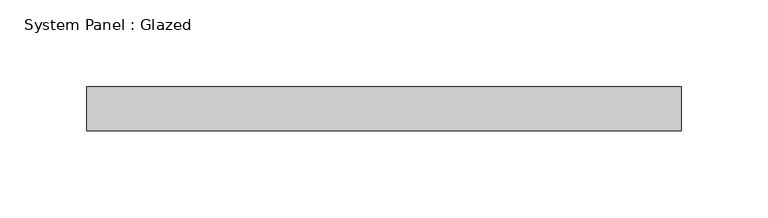
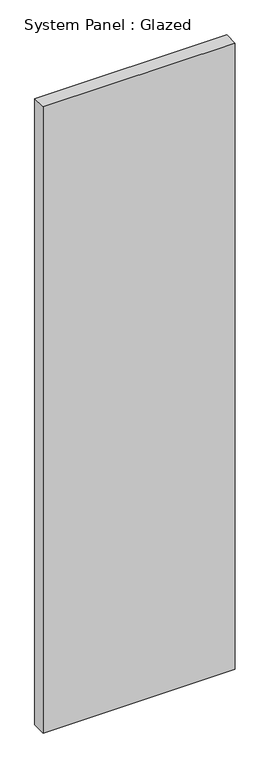
"""IFC4 building model written with IfcOpenShell, lengths in millimetres: plate geometry, System Panel : Glazed."""

from ifc_helpers import new_model, si_unit, origin, origin_with_axes, place, context, project, spatial, polyline, outline, extrude, source, transform, mapped, element, save


def system_panel_glazed_bd2ad356(model_context):
    return source(origin(), model_context, "Body", "SweptSolid", [
        extrude(outline(polyline([(171.45, 19.05), (-171.45, 19.05), (-171.45, 44.45), (171.45, 44.45), (171.45, 19.05)])), origin_with_axes(), (0.0, 0.0, 1.0), 1181.1),
    ])


if __name__ == "__main__":
    model = new_model("IFC4")
    model_context = context("Model", 3, world=origin())
    ifc_project = project(units=[si_unit("LENGTHUNIT", "METRE", prefix="MILLI")], contexts=[model_context])
    site = spatial("IfcSite", under=ifc_project)
    building = spatial("IfcBuilding", under=site)
    placement = place(None, origin())
    system_panel_glazed_shape = system_panel_glazed_bd2ad356(model_context)
    element("IfcPlate", 1, ObjectType="System Panel : Glazed", at=placement, inside=building, context=model_context, shape_type="MappedRepresentation", body=[
        mapped(system_panel_glazed_shape, transform((0.0, 0.0, 0.0), x_axis=(1.0, 0.0, 0.0), y_axis=(0.0, 1.0, 0.0), z_axis=(0.0, 0.0, 1.0))),
    ])
    save(model, "model.ifc")

# Revit data of these elements
# Type "System Panel : Glazed"
#   Construction Type Id = "GSP4R"
#   Analytic Construction = "1/8 in Pilkington single glazing"
#   Visual Light Transmittance = 0.9
#   Solar Heat Gain Coefficient = 0.86
#   Heat Transfer Coefficient (U) = 1.18115 BTU/(h·ft²·°F)
# Element 1 (IfcPlate, "System Panel : Glazed")
#   Materials on its faces: "Glass"
# Materials
#   "Glass": class "Glass", colour RGB 0 128 192, transparency 0.75, Description = "Soda Lime Glass", Cost = 0
